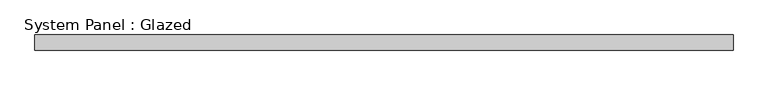
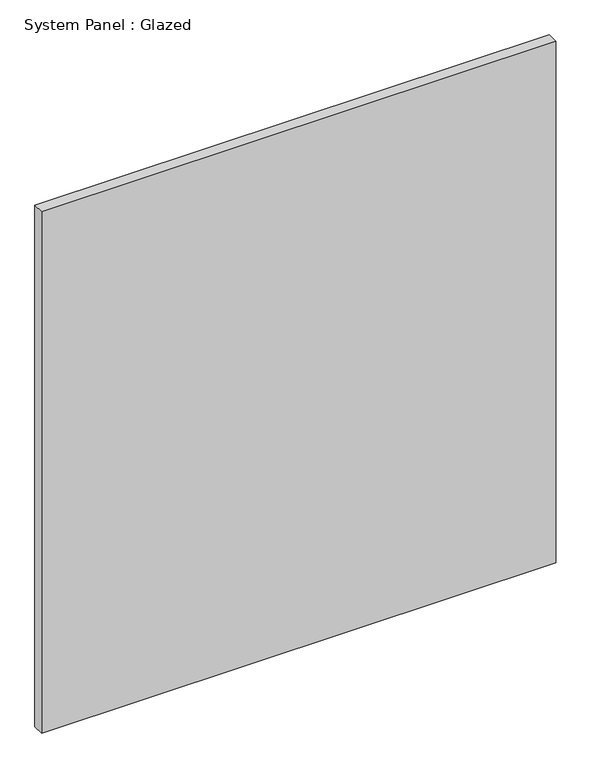
"""IFC4 building model written with IfcOpenShell, lengths in millimetres: plate geometry, System Panel : Glazed."""

from ifc_helpers import new_model, si_unit, origin, origin_with_axes, place, context, project, spatial, polyline, outline, extrude, source, transform, mapped, element, save


def system_panel_glazed_c4c31c98(model_context):
    return source(origin(), model_context, "Body", "SweptSolid", [
        extrude(outline(polyline([(568.8014963, 19.05), (-568.8014963, 19.05), (-568.8014963, 44.45), (568.8014963, 44.45), (568.8014963, 19.05)])), origin_with_axes(), (0.0, 0.0, 1.0), 1219.2),
    ])


if __name__ == "__main__":
    model = new_model("IFC4")
    model_context = context("Model", 3, world=origin())
    ifc_project = project(units=[si_unit("LENGTHUNIT", "METRE", prefix="MILLI")], contexts=[model_context])
    site = spatial("IfcSite", under=ifc_project)
    building = spatial("IfcBuilding", under=site)
    placement = place(None, origin())
    system_panel_glazed_shape = system_panel_glazed_c4c31c98(model_context)
    element("IfcPlate", 1, ObjectType="System Panel : Glazed", at=placement, inside=building, context=model_context, shape_type="MappedRepresentation", body=[
        mapped(system_panel_glazed_shape, transform((0.0, 0.0, 0.0), x_axis=(1.0, 0.0, 0.0), y_axis=(0.0, 1.0, 0.0), z_axis=(0.0, 0.0, 1.0))),
    ])
    save(model, "model.ifc")

# Revit data of these elements
# Type "System Panel : Glazed"
#   Construction Type Id = "GSP4R"
#   Analytic Construction = "1/8 in Pilkington single glazing"
#   Visual Light Transmittance = 0.9
#   Solar Heat Gain Coefficient = 0.86
#   Heat Transfer Coefficient (U) = 1.18115 BTU/(h·ft²·°F)
# Element 1 (IfcPlate, "System Panel : Glazed")
#   Materials on its faces: "Glass"
# Materials
#   "Glass": class "Glass", colour RGB 0 128 192, transparency 0.75, Description = "Soda Lime Glass", Cost = 0
